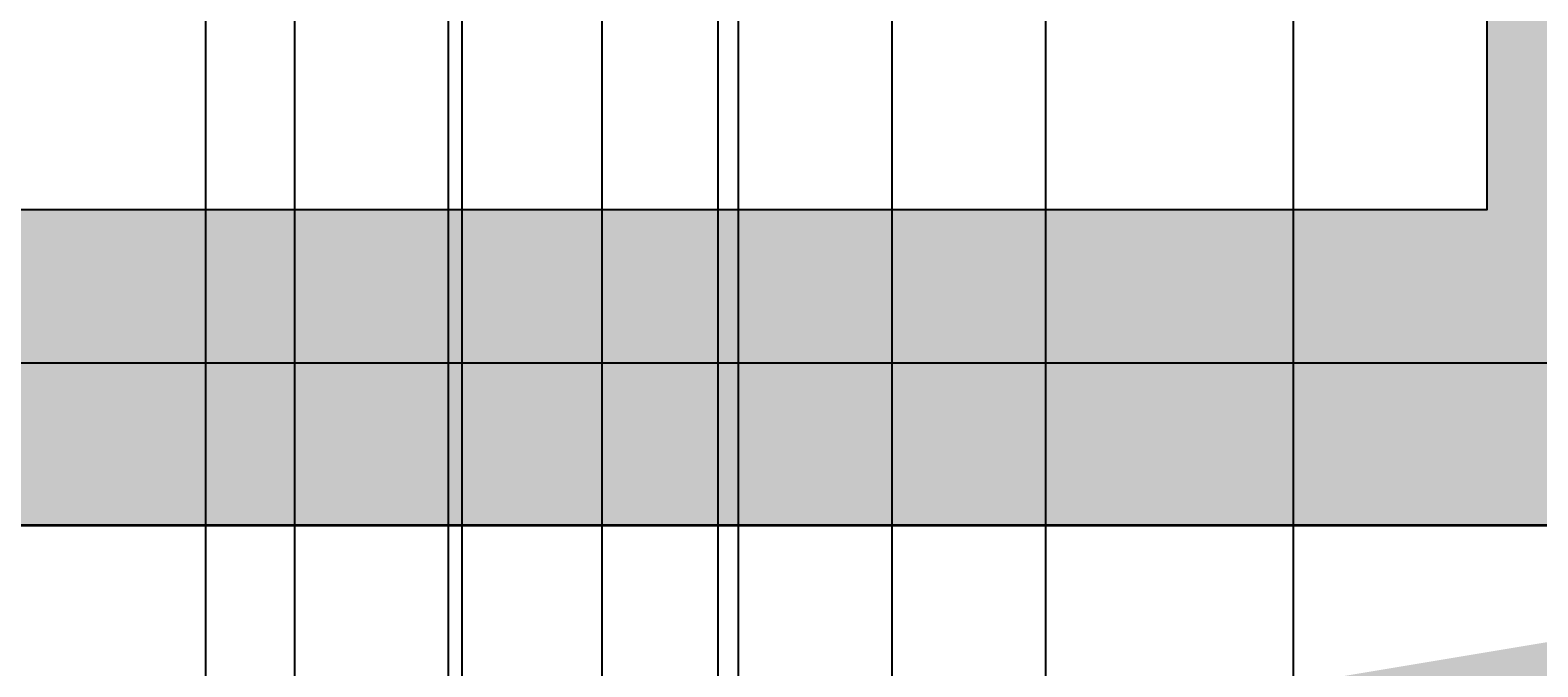
# Model space of a CAD drawing. Units: millimetres. Extents: x -22994 to 29398, y -19990 to 20176.
# Tile 33 of 135: x 139 to 198, y 5 to 30. Entities that reach past the tile are written whole.
import ezdxf
from ezdxf import colors
from ezdxf.entities.mleader import LeaderData, LeaderLine
from ezdxf.math import Vec2, Vec3

# ---------------------------------------------------------------- set-up
doc = ezdxf.new("R2010")
doc.units = ezdxf.units.MM
doc.header["$MEASUREMENT"] = 0
for name, color, linetype, lineweight in [('M-ANNO-TEXT', 7, 'Continuous', 25), ('M-DIMS', 2, 'Continuous', 18), ('M-EQPM', 7, 'Continuous', 25), ('M-EQPM-PATT', 7, 'Continuous', 18), ('S-FNDN', 7, 'Continuous', 35)]:
    doc.layers.add(name, color=color, linetype=linetype, lineweight=lineweight)
doc.styles.get("Standard").update_dxf_attribs({"font": 'arial.ttf'})
doc.dimstyles.get("Standard").update_dxf_attribs({"dimtxt": 0.18, "dimasz": 10000, "dimexe": 0.18, "dimexo": 0.0625, "dimgap": 0.09, "dimtad": 0, "dimtih": 1, "dimtoh": 1, "dimdec": 0, "dimzin": 0, "dimdsep": 46, "dimtxsty": 'Standard', "dimcen": 0.09, "dimadec": 0, "dimazin": 0, "dimtfac": 1, "dimtdec": 0, "dimtofl": 0, "dimtmove": 0, "dimatfit": 3, "dimfxl": 1, "dimtolj": 1, "dimtzin": 0, "dimlwd": 30, "dimarcsym": 0})

# ---------------------------------------------------------------- blocks, each defined once
blk = doc.blocks.new('*D2')
at = {"layer": 'Defpoints', "color": 0, "transparency": 16777216}
for p in [(6.677, 10.271), (290.852, 10.271), (290.852, -5.079)]:
    blk.add_point(p, dxfattribs=at)
at = {"layer": 'M-DIMS', "color": 0, "lineweight": -2, "transparency": 16777216}
for p, q in [((6.677, 10.209), (6.677, -5.259)), ((290.852, 10.209), (290.852, -5.259))]:
    blk.add_line(p, q, dxfattribs=at)
at = {"layer": 'M-DIMS', "color": 0, "lineweight": 30, "transparency": 16777216}
for p, q in [((-9993.323, -5.079), (-19993.323, -5.079)), ((10290.852, -5.079), (20290.852, -5.079))]:
    blk.add_line(p, q, dxfattribs=at)
at = {"layer": 'M-DIMS', "color": 0, "transparency": 16777216}
for points in [[(-9993.323, 1661.588), (-9993.323, -1671.745), (6.677, -5.079)], [(10290.852, 1661.588), (10290.852, -1671.745), (290.852, -5.079)]]:
    blk.add_solid(points, dxfattribs=at)
at = {"layer": 'M-DIMS', "color": 0, "transparency": 16777216, "insert": (148.765, -5.079), "char_height": 0.18, "attachment_point": 5}
blk.add_mtext('\\A1;284.2', dxfattribs=at)
blk = doc.blocks.new('*D3')
at = {"layer": 'Defpoints', "color": 0, "transparency": 16777216}
for p in [(110.265, 204.165), (110.265, 176.366), (95.833, 127.967)]:
    blk.add_point(p, dxfattribs=at)
at = {"layer": 'M-DIMS', "color": 0, "lineweight": -2, "transparency": 16777216}
for p, q in [((95.833, 128.03), (95.833, 204.345)), ((110.265, 176.429), (110.265, 204.345))]:
    blk.add_line(p, q, dxfattribs=at)
at = {"layer": 'M-DIMS', "color": 0, "lineweight": 30, "transparency": 16777216}
for p, q in [((-9904.167, 204.165), (-19904.167, 204.165)), ((10110.265, 204.165), (20110.265, 204.165))]:
    blk.add_line(p, q, dxfattribs=at)
at = {"layer": 'M-DIMS', "color": 0, "transparency": 16777216}
for points in [[(-9904.167, 1870.832), (-9904.167, -1462.501), (95.833, 204.165)], [(10110.265, 1870.832), (10110.265, -1462.501), (110.265, 204.165)]]:
    blk.add_solid(points, dxfattribs=at)
at = {"layer": 'M-DIMS', "color": 0, "transparency": 16777216, "insert": (103.049, 204.165), "char_height": 0.18, "attachment_point": 5}
blk.add_mtext('\\A1;14.432', dxfattribs=at)
blk = doc.blocks.new('*D4')
at = {"layer": 'Defpoints', "color": 0, "transparency": 16777216}
for p in [(116.265, 204.165), (110.265, 176.366), (116.265, 176.366)]:
    blk.add_point(p, dxfattribs=at)
at = {"layer": 'M-DIMS', "color": 0, "lineweight": -2, "transparency": 16777216}
for p, q in [((110.265, 176.429), (110.265, 204.345)), ((116.265, 176.429), (116.265, 204.345))]:
    blk.add_line(p, q, dxfattribs=at)
at = {"layer": 'M-DIMS', "color": 0, "lineweight": 30, "transparency": 16777216}
for p, q in [((-9889.735, 204.165), (-19889.735, 204.165)), ((10116.265, 204.165), (20116.265, 204.165))]:
    blk.add_line(p, q, dxfattribs=at)
at = {"layer": 'M-DIMS', "color": 0, "transparency": 16777216}
for points in [[(-9889.735, 1870.832), (-9889.735, -1462.501), (110.265, 204.165)], [(10116.265, 1870.832), (10116.265, -1462.501), (116.265, 204.165)]]:
    blk.add_solid(points, dxfattribs=at)
at = {"layer": 'M-DIMS', "color": 0, "transparency": 16777216, "insert": (113.265, 204.165), "char_height": 0.18, "attachment_point": 5}
blk.add_mtext('\\A1;6', dxfattribs=at)
blk = doc.blocks.new('*D5')
at = {"layer": 'Defpoints', "color": 0, "transparency": 16777216}
for p in [(181.265, 204.165), (116.265, 176.366), (181.265, 176.366)]:
    blk.add_point(p, dxfattribs=at)
at = {"layer": 'M-DIMS', "color": 0, "lineweight": -2, "transparency": 16777216}
for p, q in [((116.265, 176.429), (116.265, 204.345)), ((181.265, 176.429), (181.265, 204.345))]:
    blk.add_line(p, q, dxfattribs=at)
at = {"layer": 'M-DIMS', "color": 0, "lineweight": 30, "transparency": 16777216}
for p, q in [((-9883.735, 204.165), (-19883.735, 204.165)), ((10181.265, 204.165), (20181.265, 204.165))]:
    blk.add_line(p, q, dxfattribs=at)
at = {"layer": 'M-DIMS', "color": 0, "transparency": 16777216}
for points in [[(-9883.735, 1870.832), (-9883.735, -1462.501), (116.265, 204.165)], [(10181.265, 1870.832), (10181.265, -1462.501), (181.265, 204.165)]]:
    blk.add_solid(points, dxfattribs=at)
at = {"layer": 'M-DIMS', "color": 0, "transparency": 16777216, "insert": (148.765, 204.165), "char_height": 0.18, "attachment_point": 5}
blk.add_mtext('\\A1;65', dxfattribs=at)
blk = doc.blocks.new('*D6')
at = {"layer": 'Defpoints', "color": 0, "transparency": 16777216}
for p in [(187.265, 204.165), (181.265, 176.366), (187.265, 176.366)]:
    blk.add_point(p, dxfattribs=at)
at = {"layer": 'M-DIMS', "color": 0, "lineweight": -2, "transparency": 16777216}
for p, q in [((181.265, 176.429), (181.265, 204.345)), ((187.265, 176.429), (187.265, 204.345))]:
    blk.add_line(p, q, dxfattribs=at)
at = {"layer": 'M-DIMS', "color": 0, "lineweight": 30, "transparency": 16777216}
for p, q in [((-9818.735, 204.165), (-19818.735, 204.165)), ((10187.265, 204.165), (20187.265, 204.165))]:
    blk.add_line(p, q, dxfattribs=at)
at = {"layer": 'M-DIMS', "color": 0, "transparency": 16777216}
for points in [[(-9818.735, 1870.832), (-9818.735, -1462.501), (181.265, 204.165)], [(10187.265, 1870.832), (10187.265, -1462.501), (187.265, 204.165)]]:
    blk.add_solid(points, dxfattribs=at)
at = {"layer": 'M-DIMS', "color": 0, "transparency": 16777216, "insert": (184.265, 204.165), "char_height": 0.18, "attachment_point": 5}
blk.add_mtext('\\A1;6', dxfattribs=at)
blk = doc.blocks.new('*D7')
at = {"layer": 'Defpoints', "color": 0, "transparency": 16777216}
for p in [(201.697, 204.165), (187.265, 176.366), (201.697, 127.967)]:
    blk.add_point(p, dxfattribs=at)
at = {"layer": 'M-DIMS', "color": 0, "lineweight": -2, "transparency": 16777216}
for p, q in [((187.265, 176.429), (187.265, 204.345)), ((201.697, 128.03), (201.697, 204.345))]:
    blk.add_line(p, q, dxfattribs=at)
at = {"layer": 'M-DIMS', "color": 0, "lineweight": 30, "transparency": 16777216}
for p, q in [((-9812.735, 204.165), (-19812.735, 204.165)), ((10201.697, 204.165), (20201.697, 204.165))]:
    blk.add_line(p, q, dxfattribs=at)
at = {"layer": 'M-DIMS', "color": 0, "transparency": 16777216}
for points in [[(-9812.735, 1870.832), (-9812.735, -1462.501), (187.265, 204.165)], [(10201.697, 1870.832), (10201.697, -1462.501), (201.697, 204.165)]]:
    blk.add_solid(points, dxfattribs=at)
at = {"layer": 'M-DIMS', "color": 0, "transparency": 16777216, "insert": (194.481, 204.165), "char_height": 0.18, "attachment_point": 5}
blk.add_mtext('\\A1;14.432', dxfattribs=at)
blk = doc.blocks.new('*D8')
at = {"layer": 'Defpoints', "color": 0, "transparency": 16777216}
for p in [(227.648, 204.165), (227.648, 146.73), (201.697, 127.967)]:
    blk.add_point(p, dxfattribs=at)
at = {"layer": 'M-DIMS', "color": 0, "lineweight": -2, "transparency": 16777216}
for p, q in [((201.697, 128.03), (201.697, 204.345)), ((227.648, 146.792), (227.648, 204.345))]:
    blk.add_line(p, q, dxfattribs=at)
at = {"layer": 'M-DIMS', "color": 0, "lineweight": 30, "transparency": 16777216}
for p, q in [((-9798.303, 204.165), (-19798.303, 204.165)), ((10227.648, 204.165), (20227.648, 204.165))]:
    blk.add_line(p, q, dxfattribs=at)
at = {"layer": 'M-DIMS', "color": 0, "transparency": 16777216}
for points in [[(-9798.303, 1870.832), (-9798.303, -1462.501), (201.697, 204.165)], [(10227.648, 1870.832), (10227.648, -1462.501), (227.648, 204.165)]]:
    blk.add_solid(points, dxfattribs=at)
at = {"layer": 'M-DIMS', "color": 0, "transparency": 16777216, "insert": (214.673, 204.165), "char_height": 0.18, "attachment_point": 5}
blk.add_mtext('\\A1;25.95', dxfattribs=at)
blk = doc.blocks.new('*D9')
at = {"layer": 'Defpoints', "color": 0, "transparency": 16777216}
for p in [(187.265, 176.366), (306.202, 176.366), (290.852, 10.271)]:
    blk.add_point(p, dxfattribs=at)
at = {"layer": 'M-DIMS', "color": 0, "lineweight": 30, "transparency": 16777216}
for p, q in [((306.202, 10176.366), (306.202, 20176.366)), ((306.202, -9989.729), (306.202, -19989.729))]:
    blk.add_line(p, q, dxfattribs=at)
at = {"layer": 'M-DIMS', "color": 0, "lineweight": -2, "transparency": 16777216}
for p, q in [((187.327, 176.366), (306.382, 176.366)), ((290.915, 10.271), (306.382, 10.271))]:
    blk.add_line(p, q, dxfattribs=at)
at = {"layer": 'M-DIMS', "color": 0, "transparency": 16777216}
for points in [[(-1360.465, 10176.366), (1972.869, 10176.366), (306.202, 176.366)], [(-1360.465, -9989.729), (1972.869, -9989.729), (306.202, 10.271)]]:
    blk.add_solid(points, dxfattribs=at)
at = {"layer": 'M-DIMS', "color": 0, "transparency": 16777216, "insert": (306.202, 93.319), "char_height": 0.18, "attachment_point": 5}
blk.add_mtext('\\A1;166.1', dxfattribs=at)
blk = doc.blocks.new('*D10')
at = {"layer": 'Defpoints', "color": 0, "transparency": 16777216}
for p in [(125.65, 136.071), (133.346, 136.071), (133.346, -5.079)]:
    blk.add_point(p, dxfattribs=at)
at = {"layer": 'M-DIMS', "color": 0, "lineweight": -2, "transparency": 16777216}
for p, q in [((125.65, 136.009), (125.65, -5.259)), ((133.346, 136.009), (133.346, -5.259))]:
    blk.add_line(p, q, dxfattribs=at)
at = {"layer": 'M-DIMS', "color": 0, "lineweight": 30, "transparency": 16777216}
for p, q in [((-9874.35, -5.079), (-19874.35, -5.079)), ((10133.346, -5.079), (20133.346, -5.079))]:
    blk.add_line(p, q, dxfattribs=at)
at = {"layer": 'M-DIMS', "color": 0, "transparency": 16777216}
for points in [[(-9874.35, 1661.588), (-9874.35, -1671.745), (125.65, -5.079)], [(10133.346, 1661.588), (10133.346, -1671.745), (133.346, -5.079)]]:
    blk.add_solid(points, dxfattribs=at)
at = {"layer": 'M-DIMS', "color": 0, "transparency": 16777216, "insert": (129.498, -5.079), "char_height": 0.18, "attachment_point": 5}
blk.add_mtext('\\A1;7.696', dxfattribs=at)
blk = doc.blocks.new('*D11')
at = {"layer": 'Defpoints', "color": 0, "transparency": 16777216}
for p in [(133.346, 136.071), (135.65, 136.071), (135.65, -5.079)]:
    blk.add_point(p, dxfattribs=at)
at = {"layer": 'M-DIMS', "color": 0, "lineweight": -2, "transparency": 16777216}
for p, q in [((133.346, 136.009), (133.346, -5.259)), ((135.65, 136.009), (135.65, -5.259))]:
    blk.add_line(p, q, dxfattribs=at)
at = {"layer": 'M-DIMS', "color": 0, "lineweight": 30, "transparency": 16777216}
for p, q in [((-9866.654, -5.079), (-19866.654, -5.079)), ((10135.65, -5.079), (20135.65, -5.079))]:
    blk.add_line(p, q, dxfattribs=at)
at = {"layer": 'M-DIMS', "color": 0, "transparency": 16777216}
for points in [[(-9866.654, 1661.588), (-9866.654, -1671.745), (133.346, -5.079)], [(10135.65, 1661.588), (10135.65, -1671.745), (135.65, -5.079)]]:
    blk.add_solid(points, dxfattribs=at)
at = {"layer": 'M-DIMS', "color": 0, "transparency": 16777216, "insert": (134.498, -5.079), "char_height": 0.18, "attachment_point": 5}
blk.add_mtext('\\A1;2.304', dxfattribs=at)
blk = doc.blocks.new('*D12')
at = {"layer": 'Defpoints', "color": 0, "transparency": 16777216}
for p in [(135.65, 136.071), (145.65, 136.071), (145.65, -5.079)]:
    blk.add_point(p, dxfattribs=at)
at = {"layer": 'M-DIMS', "color": 0, "lineweight": -2, "transparency": 16777216}
for p, q in [((135.65, 136.009), (135.65, -5.259)), ((145.65, 136.009), (145.65, -5.259))]:
    blk.add_line(p, q, dxfattribs=at)
at = {"layer": 'M-DIMS', "color": 0, "lineweight": 30, "transparency": 16777216}
for p, q in [((-9864.35, -5.079), (-19864.35, -5.079)), ((10145.65, -5.079), (20145.65, -5.079))]:
    blk.add_line(p, q, dxfattribs=at)
at = {"layer": 'M-DIMS', "color": 0, "transparency": 16777216}
for points in [[(-9864.35, 1661.588), (-9864.35, -1671.745), (135.65, -5.079)], [(10145.65, 1661.588), (10145.65, -1671.745), (145.65, -5.079)]]:
    blk.add_solid(points, dxfattribs=at)
at = {"layer": 'M-DIMS', "color": 0, "transparency": 16777216, "insert": (140.65, -5.079), "char_height": 0.18, "attachment_point": 5}
blk.add_mtext('\\A1;10', dxfattribs=at)
blk = doc.blocks.new('*D13')
at = {"layer": 'Defpoints', "color": 0, "transparency": 16777216}
for p in [(145.65, 136.071), (155.65, 136.071), (155.65, -5.079)]:
    blk.add_point(p, dxfattribs=at)
at = {"layer": 'M-DIMS', "color": 0, "lineweight": -2, "transparency": 16777216}
for p, q in [((145.65, 136.009), (145.65, -5.259)), ((155.65, 136.009), (155.65, -5.259))]:
    blk.add_line(p, q, dxfattribs=at)
at = {"layer": 'M-DIMS', "color": 0, "lineweight": 30, "transparency": 16777216}
for p, q in [((-9854.35, -5.079), (-19854.35, -5.079)), ((10155.65, -5.079), (20155.65, -5.079))]:
    blk.add_line(p, q, dxfattribs=at)
at = {"layer": 'M-DIMS', "color": 0, "transparency": 16777216}
for points in [[(-9854.35, 1661.588), (-9854.35, -1671.745), (145.65, -5.079)], [(10155.65, 1661.588), (10155.65, -1671.745), (155.65, -5.079)]]:
    blk.add_solid(points, dxfattribs=at)
at = {"layer": 'M-DIMS', "color": 0, "transparency": 16777216, "insert": (150.65, -5.079), "char_height": 0.18, "attachment_point": 5}
blk.add_mtext('\\A1;10', dxfattribs=at)
blk = doc.blocks.new('*D14')
at = {"layer": 'Defpoints', "color": 0, "transparency": 16777216}
for p in [(155.65, 136.071), (165.65, 136.071), (165.65, -5.079)]:
    blk.add_point(p, dxfattribs=at)
at = {"layer": 'M-DIMS', "color": 0, "lineweight": -2, "transparency": 16777216}
for p, q in [((155.65, 136.009), (155.65, -5.259)), ((165.65, 136.009), (165.65, -5.259))]:
    blk.add_line(p, q, dxfattribs=at)
at = {"layer": 'M-DIMS', "color": 0, "lineweight": 30, "transparency": 16777216}
for p, q in [((-9844.35, -5.079), (-19844.35, -5.079)), ((10165.65, -5.079), (20165.65, -5.079))]:
    blk.add_line(p, q, dxfattribs=at)
at = {"layer": 'M-DIMS', "color": 0, "transparency": 16777216}
for points in [[(-9844.35, 1661.588), (-9844.35, -1671.745), (155.65, -5.079)], [(10165.65, 1661.588), (10165.65, -1671.745), (165.65, -5.079)]]:
    blk.add_solid(points, dxfattribs=at)
at = {"layer": 'M-DIMS', "color": 0, "transparency": 16777216, "insert": (160.65, -5.079), "char_height": 0.18, "attachment_point": 5}
blk.add_mtext('\\A1;10', dxfattribs=at)
blk = doc.blocks.new('*D15')
at = {"layer": 'Defpoints', "color": 0, "transparency": 16777216}
for p in [(173.346, 154.788), (173.346, 136.071), (306.202, 136.071)]:
    blk.add_point(p, dxfattribs=at)
at = {"layer": 'M-DIMS', "color": 0, "lineweight": 30, "transparency": 16777216}
for p, q in [((306.202, 10154.788), (306.202, 20154.788)), ((306.202, -9863.929), (306.202, -19863.929))]:
    blk.add_line(p, q, dxfattribs=at)
at = {"layer": 'M-DIMS', "color": 0, "lineweight": -2, "transparency": 16777216}
for p, q in [((173.408, 154.788), (306.382, 154.788)), ((173.408, 136.071), (306.382, 136.071))]:
    blk.add_line(p, q, dxfattribs=at)
at = {"layer": 'M-DIMS', "color": 0, "transparency": 16777216}
for points in [[(-1360.465, 10154.788), (1972.869, 10154.788), (306.202, 154.788)], [(-1360.465, -9863.929), (1972.869, -9863.929), (306.202, 136.071)]]:
    blk.add_solid(points, dxfattribs=at)
at = {"layer": 'M-DIMS', "color": 0, "transparency": 16777216, "insert": (306.202, 145.43), "char_height": 0.18, "attachment_point": 5}
blk.add_mtext('\\A1;18.717', dxfattribs=at)
blk = doc.blocks.new('*D16')
at = {"layer": 'Defpoints', "color": 0, "transparency": 16777216}
for p in [(120.17, 204.165), (110.466, 48.035), (120.17, 48.035)]:
    blk.add_point(p, dxfattribs=at)
at = {"layer": 'M-DIMS', "color": 0, "lineweight": -2, "transparency": 16777216}
for p, q in [((110.466, 48.097), (110.466, 204.345)), ((120.17, 48.097), (120.17, 204.345))]:
    blk.add_line(p, q, dxfattribs=at)
at = {"layer": 'M-DIMS', "color": 0, "lineweight": 30, "transparency": 16777216}
for p, q in [((-9889.534, 204.165), (-19889.534, 204.165)), ((10120.17, 204.165), (20120.17, 204.165))]:
    blk.add_line(p, q, dxfattribs=at)
at = {"layer": 'M-DIMS', "color": 0, "transparency": 16777216}
for points in [[(-9889.534, 1870.832), (-9889.534, -1462.501), (110.466, 204.165)], [(10120.17, 1870.832), (10120.17, -1462.501), (120.17, 204.165)]]:
    blk.add_solid(points, dxfattribs=at)
at = {"layer": 'M-DIMS', "color": 0, "transparency": 16777216, "insert": (115.318, 204.165), "char_height": 0.18, "attachment_point": 5}
blk.add_mtext('\\A1;9.704', dxfattribs=at)
blk = doc.blocks.new('*D17')
at = {"layer": 'Defpoints', "color": 0, "transparency": 16777216}
for p in [(126.17, 204.165), (120.17, 48.035), (126.17, 48.035)]:
    blk.add_point(p, dxfattribs=at)
at = {"layer": 'M-DIMS', "color": 0, "lineweight": -2, "transparency": 16777216}
for p, q in [((120.17, 48.097), (120.17, 204.345)), ((126.17, 48.097), (126.17, 204.345))]:
    blk.add_line(p, q, dxfattribs=at)
at = {"layer": 'M-DIMS', "color": 0, "lineweight": 30, "transparency": 16777216}
for p, q in [((-9879.83, 204.165), (-19879.83, 204.165)), ((10126.17, 204.165), (20126.17, 204.165))]:
    blk.add_line(p, q, dxfattribs=at)
at = {"layer": 'M-DIMS', "color": 0, "transparency": 16777216}
for points in [[(-9879.83, 1870.832), (-9879.83, -1462.501), (120.17, 204.165)], [(10126.17, 1870.832), (10126.17, -1462.501), (126.17, 204.165)]]:
    blk.add_solid(points, dxfattribs=at)
at = {"layer": 'M-DIMS', "color": 0, "transparency": 16777216, "insert": (123.17, 204.165), "char_height": 0.18, "attachment_point": 5}
blk.add_mtext('\\A1;6', dxfattribs=at)
blk = doc.blocks.new('*D18')
at = {"layer": 'Defpoints', "color": 0, "transparency": 16777216}
for p in [(132.17, 204.165), (126.17, 48.035), (132.17, 48.035)]:
    blk.add_point(p, dxfattribs=at)
at = {"layer": 'M-DIMS', "color": 0, "lineweight": -2, "transparency": 16777216}
for p, q in [((126.17, 48.097), (126.17, 204.345)), ((132.17, 48.097), (132.17, 204.345))]:
    blk.add_line(p, q, dxfattribs=at)
at = {"layer": 'M-DIMS', "color": 0, "lineweight": 30, "transparency": 16777216}
for p, q in [((-9873.83, 204.165), (-19873.83, 204.165)), ((10132.17, 204.165), (20132.17, 204.165))]:
    blk.add_line(p, q, dxfattribs=at)
at = {"layer": 'M-DIMS', "color": 0, "transparency": 16777216}
for points in [[(-9873.83, 1870.832), (-9873.83, -1462.501), (126.17, 204.165)], [(10132.17, 1870.832), (10132.17, -1462.501), (132.17, 204.165)]]:
    blk.add_solid(points, dxfattribs=at)
at = {"layer": 'M-DIMS', "color": 0, "transparency": 16777216, "insert": (129.17, 204.165), "char_height": 0.18, "attachment_point": 5}
blk.add_mtext('\\A1;6', dxfattribs=at)
blk = doc.blocks.new('*D19')
at = {"layer": 'Defpoints', "color": 0, "transparency": 16777216}
for p in [(138.17, 204.165), (132.17, 48.035), (138.17, 48.035)]:
    blk.add_point(p, dxfattribs=at)
at = {"layer": 'M-DIMS', "color": 0, "lineweight": -2, "transparency": 16777216}
for p, q in [((132.17, 48.097), (132.17, 204.345)), ((138.17, 48.097), (138.17, 204.345))]:
    blk.add_line(p, q, dxfattribs=at)
at = {"layer": 'M-DIMS', "color": 0, "lineweight": 30, "transparency": 16777216}
for p, q in [((-9867.83, 204.165), (-19867.83, 204.165)), ((10138.17, 204.165), (20138.17, 204.165))]:
    blk.add_line(p, q, dxfattribs=at)
at = {"layer": 'M-DIMS', "color": 0, "transparency": 16777216}
for points in [[(-9867.83, 1870.832), (-9867.83, -1462.501), (132.17, 204.165)], [(10138.17, 1870.832), (10138.17, -1462.501), (138.17, 204.165)]]:
    blk.add_solid(points, dxfattribs=at)
at = {"layer": 'M-DIMS', "color": 0, "transparency": 16777216, "insert": (135.17, 204.165), "char_height": 0.18, "attachment_point": 5}
blk.add_mtext('\\A1;6', dxfattribs=at)
blk = doc.blocks.new('*D20')
at = {"layer": 'Defpoints', "color": 0, "transparency": 16777216}
for p in [(144.17, 204.165), (138.17, 48.035), (144.17, 48.035)]:
    blk.add_point(p, dxfattribs=at)
at = {"layer": 'M-DIMS', "color": 0, "lineweight": -2, "transparency": 16777216}
for p, q in [((138.17, 48.097), (138.17, 204.345)), ((144.17, 48.097), (144.17, 204.345))]:
    blk.add_line(p, q, dxfattribs=at)
at = {"layer": 'M-DIMS', "color": 0, "lineweight": 30, "transparency": 16777216}
for p, q in [((-9861.83, 204.165), (-19861.83, 204.165)), ((10144.17, 204.165), (20144.17, 204.165))]:
    blk.add_line(p, q, dxfattribs=at)
at = {"layer": 'M-DIMS', "color": 0, "transparency": 16777216}
for points in [[(-9861.83, 1870.832), (-9861.83, -1462.501), (138.17, 204.165)], [(10144.17, 1870.832), (10144.17, -1462.501), (144.17, 204.165)]]:
    blk.add_solid(points, dxfattribs=at)
at = {"layer": 'M-DIMS', "color": 0, "transparency": 16777216, "insert": (141.17, 204.165), "char_height": 0.18, "attachment_point": 5}
blk.add_mtext('\\A1;6', dxfattribs=at)
blk = doc.blocks.new('*D21')
at = {"layer": 'Defpoints', "color": 0, "transparency": 16777216}
for p in [(149.116, 204.165), (144.17, 48.035), (149.116, 48.035)]:
    blk.add_point(p, dxfattribs=at)
at = {"layer": 'M-DIMS', "color": 0, "lineweight": -2, "transparency": 16777216}
for p, q in [((144.17, 48.097), (144.17, 204.345)), ((149.116, 48.097), (149.116, 204.345))]:
    blk.add_line(p, q, dxfattribs=at)
at = {"layer": 'M-DIMS', "color": 0, "lineweight": 30, "transparency": 16777216}
for p, q in [((-9855.83, 204.165), (-19855.83, 204.165)), ((10149.116, 204.165), (20149.116, 204.165))]:
    blk.add_line(p, q, dxfattribs=at)
at = {"layer": 'M-DIMS', "color": 0, "transparency": 16777216}
for points in [[(-9855.83, 1870.832), (-9855.83, -1462.501), (144.17, 204.165)], [(10149.116, 1870.832), (10149.116, -1462.501), (149.116, 204.165)]]:
    blk.add_solid(points, dxfattribs=at)
at = {"layer": 'M-DIMS', "color": 0, "transparency": 16777216, "insert": (146.643, 204.165), "char_height": 0.18, "attachment_point": 5}
blk.add_mtext('\\A1;4.945', dxfattribs=at)
blk = doc.blocks.new('*D22')
at = {"layer": 'Defpoints', "color": 0, "transparency": 16777216}
for p in [(149.116, 30.99), (155.116, 30.99), (155.116, -5.079)]:
    blk.add_point(p, dxfattribs=at)
at = {"layer": 'M-DIMS', "color": 0, "lineweight": -2, "transparency": 16777216}
for p, q in [((149.116, 30.927), (149.116, -5.259)), ((155.116, 30.927), (155.116, -5.259))]:
    blk.add_line(p, q, dxfattribs=at)
at = {"layer": 'M-DIMS', "color": 0, "lineweight": 30, "transparency": 16777216}
for p, q in [((-9850.884, -5.079), (-19850.884, -5.079)), ((10155.116, -5.079), (20155.116, -5.079))]:
    blk.add_line(p, q, dxfattribs=at)
at = {"layer": 'M-DIMS', "color": 0, "transparency": 16777216}
for points in [[(-9850.884, 1661.588), (-9850.884, -1671.745), (149.116, -5.079)], [(10155.116, 1661.588), (10155.116, -1671.745), (155.116, -5.079)]]:
    blk.add_solid(points, dxfattribs=at)
at = {"layer": 'M-DIMS', "color": 0, "transparency": 16777216, "insert": (152.116, -5.079), "char_height": 0.18, "attachment_point": 5}
blk.add_mtext('\\A1;6', dxfattribs=at)
blk = doc.blocks.new('*D23')
at = {"layer": 'Defpoints', "color": 0, "transparency": 16777216}
for p in [(155.116, 30.99), (161.116, 30.99), (161.116, -5.079)]:
    blk.add_point(p, dxfattribs=at)
at = {"layer": 'M-DIMS', "color": 0, "lineweight": -2, "transparency": 16777216}
for p, q in [((155.116, 30.927), (155.116, -5.259)), ((161.116, 30.927), (161.116, -5.259))]:
    blk.add_line(p, q, dxfattribs=at)
at = {"layer": 'M-DIMS', "color": 0, "lineweight": 30, "transparency": 16777216}
for p, q in [((-9844.884, -5.079), (-19844.884, -5.079)), ((10161.116, -5.079), (20161.116, -5.079))]:
    blk.add_line(p, q, dxfattribs=at)
at = {"layer": 'M-DIMS', "color": 0, "transparency": 16777216}
for points in [[(-9844.884, 1661.588), (-9844.884, -1671.745), (155.116, -5.079)], [(10161.116, 1661.588), (10161.116, -1671.745), (161.116, -5.079)]]:
    blk.add_solid(points, dxfattribs=at)
at = {"layer": 'M-DIMS', "color": 0, "transparency": 16777216, "insert": (158.116, -5.079), "char_height": 0.18, "attachment_point": 5}
blk.add_mtext('\\A1;6', dxfattribs=at)
blk = doc.blocks.new('*D24')
at = {"layer": 'Defpoints', "color": 0, "transparency": 16777216}
for p in [(161.116, 30.99), (166.439, 30.99), (166.439, -5.079)]:
    blk.add_point(p, dxfattribs=at)
at = {"layer": 'M-DIMS', "color": 0, "lineweight": -2, "transparency": 16777216}
for p, q in [((161.116, 30.927), (161.116, -5.259)), ((166.439, 30.927), (166.439, -5.259))]:
    blk.add_line(p, q, dxfattribs=at)
at = {"layer": 'M-DIMS', "color": 0, "lineweight": 30, "transparency": 16777216}
for p, q in [((-9838.884, -5.079), (-19838.884, -5.079)), ((10166.439, -5.079), (20166.439, -5.079))]:
    blk.add_line(p, q, dxfattribs=at)
at = {"layer": 'M-DIMS', "color": 0, "transparency": 16777216}
for points in [[(-9838.884, 1661.588), (-9838.884, -1671.745), (161.116, -5.079)], [(10166.439, 1661.588), (10166.439, -1671.745), (166.439, -5.079)]]:
    blk.add_solid(points, dxfattribs=at)
at = {"layer": 'M-DIMS', "color": 0, "transparency": 16777216, "insert": (163.777, -5.079), "char_height": 0.18, "attachment_point": 5}
blk.add_mtext('\\A1;5.323', dxfattribs=at)
blk = doc.blocks.new('*D25')
at = {"layer": 'Defpoints', "color": 0, "transparency": 16777216}
for p in [(166.439, 30.99), (172.439, 30.99), (172.439, -5.079)]:
    blk.add_point(p, dxfattribs=at)
at = {"layer": 'M-DIMS', "color": 0, "lineweight": -2, "transparency": 16777216}
for p, q in [((166.439, 30.927), (166.439, -5.259)), ((172.439, 30.927), (172.439, -5.259))]:
    blk.add_line(p, q, dxfattribs=at)
at = {"layer": 'M-DIMS', "color": 0, "lineweight": 30, "transparency": 16777216}
for p, q in [((-9833.561, -5.079), (-19833.561, -5.079)), ((10172.439, -5.079), (20172.439, -5.079))]:
    blk.add_line(p, q, dxfattribs=at)
at = {"layer": 'M-DIMS', "color": 0, "transparency": 16777216}
for points in [[(-9833.561, 1661.588), (-9833.561, -1671.745), (166.439, -5.079)], [(10172.439, 1661.588), (10172.439, -1671.745), (172.439, -5.079)]]:
    blk.add_solid(points, dxfattribs=at)
at = {"layer": 'M-DIMS', "color": 0, "transparency": 16777216, "insert": (169.439, -5.079), "char_height": 0.18, "attachment_point": 5}
blk.add_mtext('\\A1;6', dxfattribs=at)
blk = doc.blocks.new('*D26')
at = {"layer": 'Defpoints', "color": 0, "transparency": 16777216}
for p in [(172.439, 30.99), (178.439, 30.99), (178.439, -5.079)]:
    blk.add_point(p, dxfattribs=at)
at = {"layer": 'M-DIMS', "color": 0, "lineweight": -2, "transparency": 16777216}
for p, q in [((172.439, 30.927), (172.439, -5.259)), ((178.439, 30.927), (178.439, -5.259))]:
    blk.add_line(p, q, dxfattribs=at)
at = {"layer": 'M-DIMS', "color": 0, "lineweight": 30, "transparency": 16777216}
for p, q in [((-9827.561, -5.079), (-19827.561, -5.079)), ((10178.439, -5.079), (20178.439, -5.079))]:
    blk.add_line(p, q, dxfattribs=at)
at = {"layer": 'M-DIMS', "color": 0, "transparency": 16777216}
for points in [[(-9827.561, 1661.588), (-9827.561, -1671.745), (172.439, -5.079)], [(10178.439, 1661.588), (10178.439, -1671.745), (178.439, -5.079)]]:
    blk.add_solid(points, dxfattribs=at)
at = {"layer": 'M-DIMS', "color": 0, "transparency": 16777216, "insert": (175.439, -5.079), "char_height": 0.18, "attachment_point": 5}
blk.add_mtext('\\A1;6', dxfattribs=at)
blk = doc.blocks.new('*D27')
at = {"layer": 'Defpoints', "color": 0, "transparency": 16777216}
for p in [(178.439, 30.99), (188.117, 30.99), (188.117, -5.079)]:
    blk.add_point(p, dxfattribs=at)
at = {"layer": 'M-DIMS', "color": 0, "lineweight": -2, "transparency": 16777216}
for p, q in [((178.439, 30.927), (178.439, -5.259)), ((188.117, 30.927), (188.117, -5.259))]:
    blk.add_line(p, q, dxfattribs=at)
at = {"layer": 'M-DIMS', "color": 0, "lineweight": 30, "transparency": 16777216}
for p, q in [((-9821.561, -5.079), (-19821.561, -5.079)), ((10188.117, -5.079), (20188.117, -5.079))]:
    blk.add_line(p, q, dxfattribs=at)
at = {"layer": 'M-DIMS', "color": 0, "transparency": 16777216}
for points in [[(-9821.561, 1661.588), (-9821.561, -1671.745), (178.439, -5.079)], [(10188.117, 1661.588), (10188.117, -1671.745), (188.117, -5.079)]]:
    blk.add_solid(points, dxfattribs=at)
at = {"layer": 'M-DIMS', "color": 0, "transparency": 16777216, "insert": (183.278, -5.079), "char_height": 0.18, "attachment_point": 5}
blk.add_mtext('\\A1;9.679', dxfattribs=at)
blk = doc.blocks.new('*D28')
at = {"layer": 'Defpoints', "color": 0, "transparency": 16777216}
for p in [(188.117, 48.035), (306.202, 48.035), (188.117, 30.99)]:
    blk.add_point(p, dxfattribs=at)
at = {"layer": 'M-DIMS', "color": 0, "lineweight": 30, "transparency": 16777216}
for p, q in [((306.202, 10048.035), (306.202, 20048.035)), ((306.202, -9969.01), (306.202, -19969.01))]:
    blk.add_line(p, q, dxfattribs=at)
at = {"layer": 'M-DIMS', "color": 0, "lineweight": -2, "transparency": 16777216}
for p, q in [((188.18, 48.035), (306.382, 48.035)), ((188.18, 30.99), (306.382, 30.99))]:
    blk.add_line(p, q, dxfattribs=at)
at = {"layer": 'M-DIMS', "color": 0, "transparency": 16777216}
for points in [[(-1360.465, 10048.035), (1972.869, 10048.035), (306.202, 48.035)], [(-1360.465, -9969.01), (1972.869, -9969.01), (306.202, 30.99)]]:
    blk.add_solid(points, dxfattribs=at)
at = {"layer": 'M-DIMS', "color": 0, "transparency": 16777216, "insert": (306.202, 39.512), "char_height": 0.18, "attachment_point": 5}
blk.add_mtext('\\A1;17.045', dxfattribs=at)
blk = doc.blocks.new('*D29')
at = {"layer": 'Defpoints', "color": 0, "transparency": 16777216}
for p in [(36.801, 80.045), (64.03, 80.045)]:
    blk.add_point(p, dxfattribs=at)
at = {"layer": 'M-DIMS', "color": 0, "lineweight": -2, "transparency": 16777216}
for p, q in [((50.415, 79.955), (50.415, 80.135)), ((50.325, 80.045), (50.505, 80.045))]:
    blk.add_line(p, q, dxfattribs=at)
at = {"layer": 'M-DIMS', "color": 0, "lineweight": 30, "transparency": 16777216}
blk.add_line((20064.03, 80.03), (10064.03, 80.038), dxfattribs=at)
at = {"layer": 'M-DIMS', "color": 0, "transparency": 16777216}
blk.add_solid([(10064.031, 1746.704), (10064.028, -1586.629), (64.03, 80.045)], dxfattribs=at)
at = {"layer": 'M-DIMS', "color": 0, "transparency": 16777216, "insert": (20064.521, 80.03), "char_height": 0.18, "attachment_point": 5}
blk.add_mtext('\\A1;∅27.23', dxfattribs=at)
blk = doc.blocks.new('*D36')
at = {"layer": 'Defpoints', "color": 0, "transparency": 16777216}
for p in [(46.39, 31.303), (46.387, 26.593)]:
    blk.add_point(p, dxfattribs=at)
at = {"layer": 'M-DIMS', "color": 0, "lineweight": 30, "transparency": 16777216}
for p, q in [((57.15, 20031.301), (51.77, 10031.302)), ((10057.15, 20031.301), (57.15, 20031.301))]:
    blk.add_line(p, q, dxfattribs=at)
at = {"layer": 'M-DIMS', "color": 0, "lineweight": -2, "transparency": 16777216}
for p, q in [((46.299, 28.948), (46.479, 28.948)), ((46.389, 28.858), (46.389, 29.038))]:
    blk.add_line(p, q, dxfattribs=at)
at = {"layer": 'M-DIMS', "color": 0, "transparency": 16777216}
blk.add_solid([(-1614.896, 10032.199), (1718.436, 10030.405), (46.39, 31.303)], dxfattribs=at)
at = {"layer": 'M-DIMS', "color": 0, "transparency": 16777216, "insert": (10057.554, 20031.301), "char_height": 0.18, "attachment_point": 5}
blk.add_mtext('\\A1;∅4.71', dxfattribs=at)
blk = doc.blocks.new('*D37')
at = {"layer": 'Defpoints', "color": 0, "transparency": 16777216}
for p in [(54.834, 118.615), (59.494, 118.614)]:
    blk.add_point(p, dxfattribs=at)
at = {"layer": 'M-DIMS', "color": 0, "lineweight": -2, "transparency": 16777216}
for p, q in [((57.074, 118.614), (57.254, 118.614)), ((57.164, 118.524), (57.164, 118.704))]:
    blk.add_line(p, q, dxfattribs=at)
at = {"layer": 'M-DIMS', "color": 0, "lineweight": 30, "transparency": 16777216}
blk.add_line((20059.493, 116.253), (10059.494, 117.434), dxfattribs=at)
at = {"layer": 'M-DIMS', "color": 0, "transparency": 16777216}
blk.add_solid([(10059.69, 1784.1), (10059.297, -1549.233), (59.494, 118.614)], dxfattribs=at)
at = {"layer": 'M-DIMS', "color": 0, "transparency": 16777216, "insert": (20059.985, 116.253), "char_height": 0.18, "attachment_point": 5}
blk.add_mtext('\\A1;∅4.659', dxfattribs=at)

msp = doc.modelspace()

# ---------------------------------------------------------------- hatches: boundary and pattern name
at = {"layer": 'M-EQPM-PATT'}
h = msp.add_hatch(color=256, dxfattribs=at)
h.set_gradient(color1=(205, 32, 39), color2=(205, 32, 39), tint=1)
h.paths.add_polyline_path([(116.2647, 150.3662), (116.2647, 170.3662), (116.2647, 176.3662), (110.2647, 176.3662), (110.2647, 152.0276), (95.8327, 127.967), (95.8327, 16.6063), (201.6967, 16.6063), (201.6967, 127.967), (187.2647, 152.0276), (187.2647, 176.3662), (181.2647, 176.3662), (181.2647, 170.3662), (181.2647, 150.3662), (195.6967, 126.3055), (195.6967, 22.6063), (101.8327, 22.6063), (101.8327, 126.3055)])
h.paths.add_polyline_path([(185.2208, 88.6347), (101.8327, 88.6347), (101.8327, 87.6347), (182.8066, 87.6347), (178.7313, 83.5594), (195.6967, 83.5594), (195.6967, 84.5594), (181.1455, 84.5594)], flags=17)
h.paths.add_polyline_path([(95.8327, 88.6347), (60.9779, 88.6347, -0.0228552), (61.7178, 87.6347), (95.8327, 87.6347)])
h.paths.add_polyline_path([(215.6212, 86.5189), (215.6212, 80.5999), (220.5095, 83.5594)])
h.paths.add_polyline_path([(215.6212, 84.5594), (201.6967, 84.5594), (201.6967, 83.5594), (215.6212, 83.5594)])
h.paths.add_polyline_path([(225.3978, 86.5189), (220.5095, 83.5594), (225.3978, 80.5999)])
h.paths.add_polyline_path([(231.6256, 84.5594), (225.3978, 84.5594), (225.3978, 83.5594), (231.6256, 83.5594)])
at = {"layer": 'S-FNDN'}
h = msp.add_hatch(color=256, dxfattribs=at)
h.set_gradient(color1=(241, 235, 31), color2=(244, 238, 81), tint=1, name='CYLINDER')
h.paths.add_polyline_path([(290.852, 16.6063), (201.6967, 16.6063), (95.8327, 16.6063), (81.8485, 16.6063), (82.3691, 10.2713), (290.852, 10.2713)])
h.paths.add_polyline_path([(81.8485, 16.6063), (60.8206, 16.6063), (62.0909, 10.2713), (82.3691, 10.2713)])
h.paths.add_polyline_path([(60.8206, 16.6063), (6.6773, 16.6063), (6.6773, 10.2713), (62.0909, 10.2713)])

# ---------------------------------------------------------------- linework, layer by layer
at = {"layer": 'M-EQPM'}
msp.add_lwpolyline([(110.2647, 176.3662), (110.2647, 152.0276), (95.8327, 127.967), (95.8327, 16.6063), (201.6967, 16.6063), (201.6967, 127.967), (187.2647, 152.0276), (187.2647, 176.3662)], close=True, dxfattribs=at)
msp.add_lwpolyline([(116.2647, 170.3662), (116.2647, 150.3662), (101.8327, 126.3055), (101.8327, 22.6063), (195.6967, 22.6063), (195.6967, 126.3055), (181.2647, 150.3662), (181.2647, 170.3662)], dxfattribs=at)
at = {"layer": 'S-FNDN'}
msp.add_lwpolyline([(95.8327, 16.6063), (6.6773, 16.6063), (6.6773, 10.2713), (290.852, 10.2713), (290.852, 16.6063), (201.6967, 16.6063)], dxfattribs=at)

# ---------------------------------------------------------------- dimensions: what is measured, and where the dimension line sits
at = {"layer": 'M-DIMS'}
for base, p1, p2, override, picture, middle in [((306.202, 176.3662), (290.852, 10.2713), (187.2647, 176.3662), {"dimdec": 1, "dimlfac": 1, "dimrnd": 0, "dimzin": 0, "dimdsep": 46, "dimlunit": 2}, '*D9', (306.202, 93.3187)), ((306.202, 136.0713), (173.3459, 154.788), (173.3459, 136.0713), {"dimdec": 3, "dimlfac": 1, "dimrnd": 0, "dimzin": 0, "dimdsep": 46, "dimlunit": 2}, '*D15', (306.202, 145.4297)), ((306.202, 48.0349), (188.1175, 30.9895), (188.1175, 48.0349), {"dimdec": 3, "dimlfac": 1, "dimrnd": 0, "dimzin": 0, "dimdsep": 46, "dimlunit": 2}, '*D28', (306.202, 39.5122))]:
    dim = msp.add_linear_dim(base=base, p1=p1, p2=p2, angle=90, dimstyle='Standard', override=override, dxfattribs=at)
    dim.commit()
    dim.dimension.update_dxf_attribs({"geometry": picture, "text_midpoint": middle})
dim = msp.add_diameter_dim_2p(p1=(46.3875, 26.5934), p2=(46.39, 31.3035), dimstyle='Standard', override={"dimdec": 2, "dimlfac": 1, "dimrnd": 0, "dimzin": 0, "dimdsep": 46, "dimlunit": 2}, dxfattribs=at)
dim.commit()
dim.dimension.update_dxf_attribs({"geometry": '*D36', "text_midpoint": (10057.5542, 20031.3006), "dimtype": 163})
for base, p1, p2, override, picture, middle in [((110.2647, 204.1654), (95.8327, 127.967), (110.2647, 176.3662), {"dimdec": 3, "dimlfac": 1, "dimrnd": 0, "dimzin": 0, "dimdsep": 46, "dimlunit": 2}, '*D3', (103.0487, 204.1654)), ((116.2647, 204.1654), (110.2647, 176.3662), (116.2647, 176.3662), {"dimdec": 0, "dimlfac": 1, "dimrnd": 0, "dimzin": 0, "dimdsep": 46, "dimlunit": 2}, '*D4', (113.2647, 204.1654)), ((120.1702, 204.1654), (110.4658, 48.0349), (120.1702, 48.0349), {"dimdec": 3, "dimlfac": 1, "dimrnd": 0, "dimzin": 0, "dimdsep": 46, "dimlunit": 2}, '*D16', (115.318, 204.1654)), ((181.2647, 204.1654), (116.2647, 176.3662), (181.2647, 176.3662), {"dimdec": 0, "dimlfac": 1, "dimrnd": 0, "dimzin": 0, "dimdsep": 46, "dimlunit": 2}, '*D5', (148.7647, 204.1654)), ((126.1702, 204.1654), (120.1702, 48.0349), (126.1702, 48.0349), {"dimdec": 0, "dimlfac": 1, "dimrnd": 0, "dimzin": 0, "dimdsep": 46, "dimlunit": 2}, '*D17', (123.1702, 204.1654)), ((132.1702, 204.1654), (126.1702, 48.0349), (132.1702, 48.0349), {"dimdec": 0, "dimlfac": 1, "dimrnd": 0, "dimzin": 0, "dimdsep": 46, "dimlunit": 2}, '*D18', (129.1702, 204.1654)), ((138.1702, 204.1654), (132.1702, 48.0349), (138.1702, 48.0349), {"dimdec": 0, "dimlfac": 1, "dimrnd": 0, "dimzin": 0, "dimdsep": 46, "dimlunit": 2}, '*D19', (135.1702, 204.1654)), ((144.1702, 204.1654), (138.1702, 48.0349), (144.1702, 48.0349), {"dimdec": 0, "dimlfac": 1, "dimrnd": 0, "dimzin": 0, "dimdsep": 46, "dimlunit": 2}, '*D20', (141.1702, 204.1654)), ((149.11567, 204.16539), (144.17023, 48.03494), (149.11567, 48.03494), {"dimdec": 3, "dimlfac": 1, "dimrnd": 0, "dimzin": 0, "dimdsep": 46, "dimlunit": 2}, '*D21', (146.64295, 204.16539)), ((187.2647, 204.1654), (181.2647, 176.3662), (187.2647, 176.3662), {"dimdec": 0, "dimlfac": 1, "dimrnd": 0, "dimzin": 0, "dimdsep": 46, "dimlunit": 2}, '*D6', (184.2647, 204.1654)), ((201.6967, 204.1654), (187.2647, 176.3662), (201.6967, 127.967), {"dimdec": 3, "dimlfac": 1, "dimrnd": 0, "dimzin": 0, "dimdsep": 46, "dimlunit": 2}, '*D7', (194.4807, 204.1654)), ((227.6485, 204.1654), (201.6967, 127.967), (227.6485, 146.7296), {"dimdec": 2, "dimlfac": 1, "dimrnd": 0, "dimzin": 0, "dimdsep": 46, "dimlunit": 2}, '*D8', (214.6726, 204.1654)), ((290.852, -5.0787), (6.6773, 10.2713), (290.852, 10.2713), {"dimdec": 1, "dimlfac": 1, "dimrnd": 0, "dimzin": 0, "dimdsep": 46, "dimlunit": 2}, '*D2', (148.7647, -5.0787)), ((133.3459, -5.0787), (125.6498, 136.0713), (133.3459, 136.0713), {"dimdec": 3, "dimlfac": 1, "dimrnd": 0, "dimzin": 0, "dimdsep": 46, "dimlunit": 2}, '*D10', (129.4978, -5.0787)), ((135.6498, -5.0787), (133.3459, 136.0713), (135.6498, 136.0713), {"dimdec": 3, "dimlfac": 1, "dimrnd": 0, "dimzin": 0, "dimdsep": 46, "dimlunit": 2}, '*D11', (134.4978, -5.0787)), ((145.6498, -5.0787), (135.6498, 136.0713), (145.6498, 136.0713), {"dimdec": 0, "dimlfac": 1, "dimrnd": 0, "dimzin": 0, "dimdsep": 46, "dimlunit": 2}, '*D12', (140.6498, -5.0787)), ((155.6498, -5.0787), (145.6498, 136.0713), (155.6498, 136.0713), {"dimdec": 0, "dimlfac": 1, "dimrnd": 0, "dimzin": 0, "dimdsep": 46, "dimlunit": 2}, '*D13', (150.6498, -5.0787)), ((155.1157, -5.0787), (149.1157, 30.9895), (155.1157, 30.9895), {"dimdec": 0, "dimlfac": 1, "dimrnd": 0, "dimzin": 0, "dimdsep": 46, "dimlunit": 2}, '*D22', (152.1157, -5.0787)), ((161.1157, -5.0787), (155.1157, 30.9895), (161.1157, 30.9895), {"dimdec": 0, "dimlfac": 1, "dimrnd": 0, "dimzin": 0, "dimdsep": 46, "dimlunit": 2}, '*D23', (158.1157, -5.0787)), ((165.6498, -5.0787), (155.6498, 136.0713), (165.6498, 136.0713), {"dimdec": 0, "dimlfac": 1, "dimrnd": 0, "dimzin": 0, "dimdsep": 46, "dimlunit": 2}, '*D14', (160.6498, -5.0787)), ((166.4387, -5.0787), (161.1157, 30.9895), (166.4387, 30.9895), {"dimdec": 3, "dimlfac": 1, "dimrnd": 0, "dimzin": 0, "dimdsep": 46, "dimlunit": 2}, '*D24', (163.7772, -5.0787)), ((172.4387, -5.0787), (166.4387, 30.9895), (172.4387, 30.9895), {"dimdec": 0, "dimlfac": 1, "dimrnd": 0, "dimzin": 0, "dimdsep": 46, "dimlunit": 2}, '*D25', (169.4387, -5.0787)), ((178.4387, -5.0787), (172.4387, 30.9895), (178.4387, 30.9895), {"dimdec": 0, "dimlfac": 1, "dimrnd": 0, "dimzin": 0, "dimdsep": 46, "dimlunit": 2}, '*D26', (175.4387, -5.0787)), ((188.1175, -5.0787), (178.4387, 30.9895), (188.1175, 30.9895), {"dimdec": 3, "dimlfac": 1, "dimrnd": 0, "dimzin": 0, "dimdsep": 46, "dimlunit": 2}, '*D27', (183.2781, -5.0787))]:
    dim = msp.add_linear_dim(base=base, p1=p1, p2=p2, dimstyle='Standard', override=override, dxfattribs=at)
    dim.commit()
    dim.dimension.update_dxf_attribs({"geometry": picture, "text_midpoint": middle})
for p1, p2, override, picture, middle in [((54.8343, 118.6145), (59.4936, 118.614), {"dimdec": 3, "dimlfac": 1, "dimrnd": 0, "dimzin": 0, "dimdsep": 46, "dimlunit": 2}, '*D37', (20059.4934, 116.2531)), ((36.8006, 80.045), (64.0296, 80.045), {"dimdec": 2, "dimlfac": 1, "dimrnd": 0, "dimzin": 0, "dimdsep": 46, "dimlunit": 2}, '*D29', (20064.0296, 80.0303))]:
    dim = msp.add_diameter_dim_2p(p1=p1, p2=p2, dimstyle='Standard', override=override, dxfattribs=at)
    dim.commit()
    dim.dimension.update_dxf_attribs({"geometry": picture, "text_midpoint": middle})

# ---------------------------------------------------------------- leaders
at = {"layer": 'M-ANNO-TEXT'}
ml = msp.add_multileader_mtext('Standard', dxfattribs=at)
ml.set_content('combustion chamber', color=256)
ml.set_leader_properties()
ml.build(insert=Vec2(0, 0))
ml.multileader.update_dxf_attribs({"dogleg_length": 0.36, "arrow_head_size": 200})
ctx = ml.context
ctx.base_point, ctx.char_height, ctx.arrow_head_size, ctx.landing_gap_size, ctx.plane_origin = Vec3(215.7321, 57.9149), 3, 200, 0.09, Vec3(189.1175, 57.9149)
notes = []
notes.append((ctx, [(0, (1, 1, 0), (215.3721, 57.9149), (1, 0), 0.36, [(0, [(189.1175, 57.9149)], 0, [])])]))
ctx.mtext.insert, ctx.mtext.flow_direction = Vec3(215.8221, 59.4394), 5
for ctx, leaders in notes:
    for number, flags, end, landing, length, lines in leaders:
        leader = LeaderData()
        leader.index, (leader.has_last_leader_line, leader.has_dogleg_vector, leader.attachment_direction) = number, flags
        leader.last_leader_point, leader.dogleg_vector, leader.dogleg_length = Vec3(end), Vec3(landing), length
        for number, points, colour, breaks in lines:
            line = LeaderLine()
            line.index, line.vertices, line.color, line.breaks = number, Vec3.list(points), colors.encode_raw_color(colour), breaks
            leader.lines.append(line)
        ctx.leaders.append(leader)

doc.saveas('drawing.dxf')
